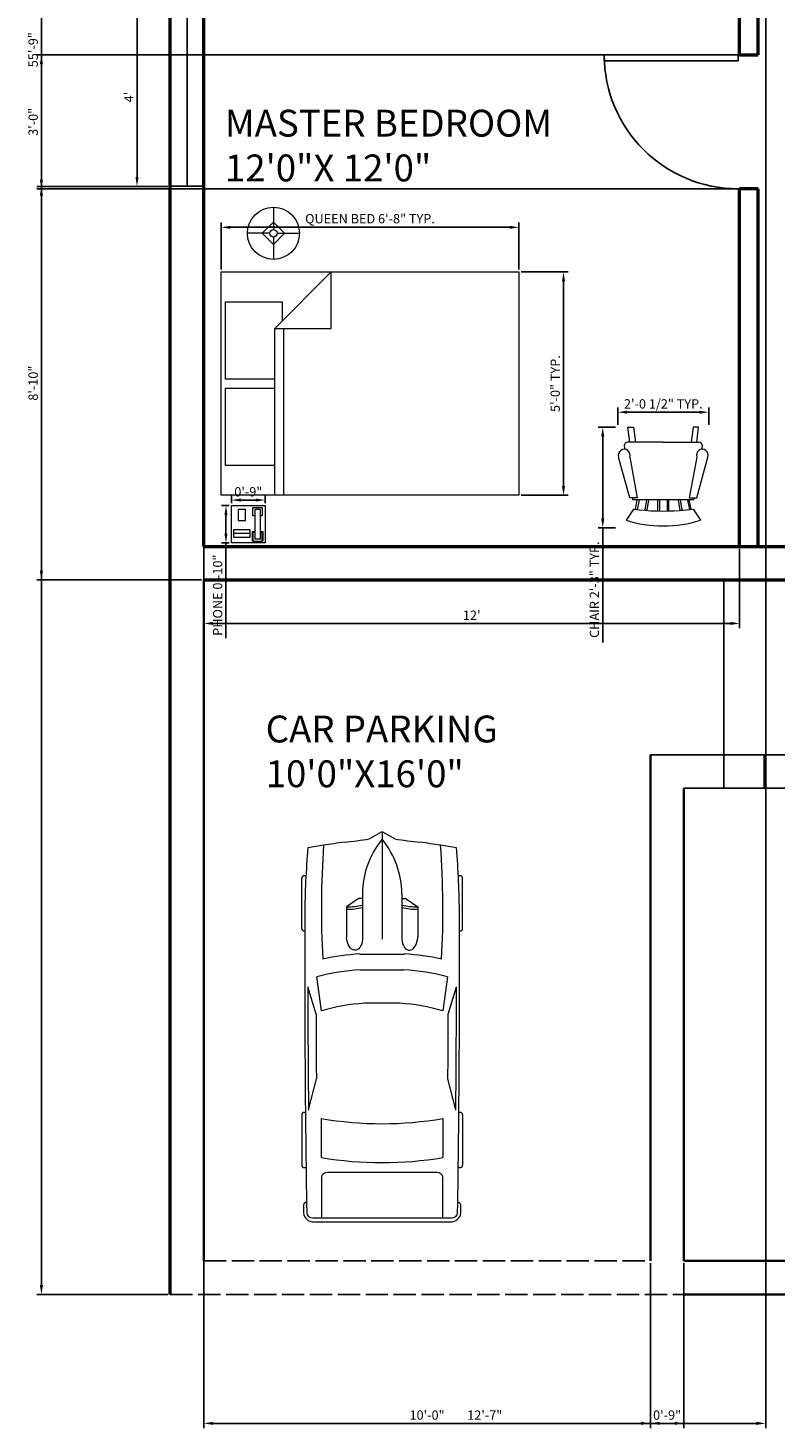
# Model space of a CAD drawing. Units: inches. Extents: x 25547 to 25983, y 30413 to 31159.
# Tile 1 of 5: x 25549 to 25750, y 30414 to 30790. Entities that reach past the tile are written whole.
import ezdxf

# ---------------------------------------------------------------- set-up
doc = ezdxf.new("R2010")
doc.units = ezdxf.units.IN
doc.linetypes.add('ACAD_ISO02W100', pattern=[15, 12, -3])
for name, color, linetype, lineweight in [('A-AREA-IDEN', 11, 'Continuous', 25), ('A-EQPM', 6, 'Continuous', 18), ('A-FLOR-PORC', 151, 'Continuous', 25), ('A-WALL', 7, 'Continuous', 50), ('C-PARK-ENTR', 7, 'ACAD_ISO02W100', 25), ('CAR', 20, 'Continuous', 13), ('DIM', 4, 'Continuous', 18), ('DOOR', 3, 'Continuous', 25), ('FURNITURES', 6, 'Continuous', 18), ('L-SITE-WALL', 7, 'Continuous', 35), ('WINDOW', 1, 'Continuous', 25)]:
    doc.layers.add(name, color=color, linetype=linetype, lineweight=lineweight)
doc.styles.get("Standard").update_dxf_attribs({"font": 'arial.ttf'})
doc.dimstyles.new('ISO-25', dxfattribs={"dimtxt": 2.5, "dimasz": 2.5, "dimexe": 1.25, "dimexo": 0.625, "dimtad": 1, "dimlunit": 3, "dimtxsty": 'Standard', "dimcen": 2.5, "dimadec": 0, "dimazin": 0, "dimtfac": 1, "dimtmove": 0, "dimatfit": 3, "dimfxl": 1, "dimarcsym": 0})

# ---------------------------------------------------------------- blocks, each defined once
blk = doc.blocks.new('*U3')
for p, q in [((0, 0), (0, -6)), ((-40, 0), (-40, -6))]:
    blk.add_line(p, q)
blk.add_lwpolyline([(0, 0), (0, 40), (-1.75, 40), (-1.75, 0)], close=True)
blk.add_arc((0, 0), 40, 90, 180)
blk = doc.blocks.new('Phone - Desk')
for p, q in [((-4.5, -5), (-4.5, 5)), ((-4.5, 5), (4.5, 5)), ((-4, 4.5), (-4, 2)), ((-3.75, 4.5), (-3.75, 2.25)), ((-1.25, 4.5), (-3.75, 4.5)), ((-3.25, 4), (-3.25, -4)), ((-3.25, 4), (-1.75, 4)), ((-1.75, -4), (-1.75, 4)), ((-1.25, 2.25), (-1.25, 4.5)), ((-1, 2), (-1, 4.5)), ((4.5, 5), (4.5, -5)), ((-4, 2), (-3.25, 2)), ((-3.75, 2.25), (-3.25, 2.25)), ((-1.75, 2.25), (-1.25, 2.25)), ((-1.75, 2), (-1, 2)), ((4, 3.5), (-0.5, 3.5)), ((-0.5, 3.5), (-0.5, 1.5)), ((-0.5, 2.5), (4, 2.5)), ((-0.5, 1.5), (4, 1.5)), ((4, 1.5), (4, 3.5)), ((-3.75, -2.25), (-3.25, -2.25)), ((-3.75, -4.5), (-3.75, -2.25)), ((-1.75, -2.25), (-1.25, -2.25)), ((-1.25, -2.25), (-1.25, -4.5)), ((2.75, -1), (0.75, -1)), ((0.75, -1), (0.75, -4)), ((2.75, -4), (2.75, -1)), ((4.5, -5), (-4.5, -5)), ((-1.25, -4.5), (-3.75, -4.5)), ((-3.25, -4), (-1.75, -4)), ((0.75, -4), (2.75, -4))]:
    blk.add_line(p, q)
blk = doc.blocks.new('Bed - Queen')
for p, q in [((0, -80.00003), (0, 0)), ((0, 0), (59.99999, 0)), ((59.99999, 0), (59.99999, -80.00003)), ((7.99999, -1.2), (28.79998, -1.2)), ((7.99999, -14.4), (7.99999, -1.2)), ((28.79998, -1.2), (28.79998, -14.4)), ((31.19999, -1.2), (51.99999, -1.2)), ((31.19999, -14.4), (31.19999, -1.2)), ((51.99999, -1.2), (51.99999, -16.4)), ((0, -14.4), (44.8, -14.4)), ((59.99999, -29.6), (44.8, -14.4)), ((44.8, -14.4), (44.8, -29.6)), ((44.8, -16.8), (0, -16.8)), ((51.99999, -16.4), (46.79936, -16.4)), ((44.8, -29.6), (59.99999, -29.6)), ((59.99999, -80.00003), (0, -80.00003))]:
    blk.add_line(p, q)
blk = doc.blocks.new('Lamp - Table')
for p, q in [((0, 7), (0, 1)), ((-1, 0), (-7, 0)), ((0, 3), (-3, 0)), ((-3, 0), (0, -3)), ((3, 0), (0, 3)), ((0, -3), (3, 0)), ((1, 0), (7, 0)), ((0, -1), (0, -7))]:
    blk.add_line(p, q)
for radius in [7, 1]:
    blk.add_circle((0, 0), radius)
blk = doc.blocks.new('Chair - Rocking')
for p, q in [((-8, -4.5), (-10, -1.5)), ((8, -4.5), (10, -1.5)), ((-9, -7.5), (-12, -18.49999)), ((-7, -7.5), (-9, -7.5)), ((-9, -18.49999), (-7, -7.5)), ((-8.23428, -6.99939), (-8.3093, -7.47958)), ((-8.23041, -7), (8.23915, -7)), ((-7.5, -4.5), (-7, -7)), ((-6.5, -7), (-7.02225, -4.43)), ((-4.5, -7), (-4.96674, -4.19951)), ((-4, -7), (-4.40532, -4.16272)), ((-1.5, -4.05012), (-1.5, -7)), ((-1, -7), (-1, -4.05012)), ((1, -7), (1, -4.04655)), ((1.5, -4.05012), (1.5, -7)), ((4, -7), (4.40187, -4.18694)), ((4.5, -7), (4.96761, -4.19437)), ((6.5, -7), (7, -4.4057)), ((7.5, -4.5), (7, -7)), ((7, -7.5), (9, -7.5)), ((9, -18.49999), (7, -7.5)), ((8.31071, -7.48854), (8.23449, -7.00073)), ((9, -7.5), (12, -18.49999)), ((-10.36644, -20.64523), (-10.5, -21.49999)), ((-9, -22.49999), (-9.5, -26.49999)), ((0, -22.49999), (-9.5, -22.49999)), ((-8, -26.49999), (-7.5, -22.49999)), ((0, -22.49999), (9.5, -22.49999)), ((8, -26.49999), (7.5, -22.49999)), ((9, -22.49999), (9.5, -26.49999)), ((10.5, -21.49999), (10.3575, -20.58798)), ((-9.5, -26.49999), (-8, -26.49999)), ((9.5, -26.49999), (8, -26.49999))]:
    blk.add_line(p, q)
for centre, radius, start, end in [((0, -34.08333), 34.08333, 72.93847, 107.0615), ((0, -68.25004), 64.25, 93.92211, 97.15267), ((0, -68.25004), 64.25, 82.84733, 93.92211), ((-10.5, -18.99999), 1.58114, 161.5651, 18.43495), ((10.5, -18.99999), 1.58114, 161.5651, 18.43495), ((-9.5, -21.49999), 1, 180, 270), ((9.5, -21.49999), 1, 270, 0)]:
    blk.add_arc(centre, radius, start, end)
blk = doc.blocks.new('*D26')
at = {"layer": 'Defpoints', "color": 0, "transparency": 16777216}
for p in [(25587.53, 30795.61), (25578.58, 30747.61), (25587.53, 30747.61)]:
    blk.add_point(p, dxfattribs=at)
at = {"layer": 'DIM', "color": 0, "lineweight": -2, "transparency": 16777216}
for p, q in [((25586.9, 30795.61), (25577.33, 30795.61)), ((25578.58, 30793.11), (25578.58, 30750.11)), ((25586.9, 30747.61), (25577.33, 30747.61))]:
    blk.add_line(p, q, dxfattribs=at)
at = {"layer": 'DIM', "color": 0, "transparency": 16777216}
for points in [[(25578.17, 30793.11), (25579, 30793.11), (25578.58, 30795.61)], [(25578.17, 30750.11), (25579, 30750.11), (25578.58, 30747.61)]]:
    blk.add_solid(points, dxfattribs=at)
at = {"layer": 'DIM', "color": 0, "transparency": 16777216, "insert": (25576.71, 30771.61), "char_height": 2.5, "attachment_point": 5, "rotation": 90}
blk.add_mtext("4'", dxfattribs=at)
blk = doc.blocks.new('*D27')
at = {"layer": 'Defpoints', "color": 0, "transparency": 16777216}
for p in [(25596.53, 30650.83), (25740.53, 30650.83), (25740.53, 30630.15)]:
    blk.add_point(p, dxfattribs=at)
at = {"layer": 'DIM', "color": 0, "lineweight": -2, "transparency": 16777216}
for p, q in [((25596.53, 30650.2), (25596.53, 30628.9)), ((25740.53, 30650.2), (25740.53, 30628.9)), ((25599.03, 30630.15), (25738.03, 30630.15))]:
    blk.add_line(p, q, dxfattribs=at)
at = {"layer": 'DIM', "color": 0, "transparency": 16777216}
for points in [[(25599.03, 30630.57), (25599.03, 30629.74), (25596.53, 30630.15)], [(25738.03, 30630.57), (25738.03, 30629.74), (25740.53, 30630.15)]]:
    blk.add_solid(points, dxfattribs=at)
at = {"layer": 'DIM', "color": 0, "transparency": 16777216, "insert": (25668.53, 30632.03), "char_height": 2.5, "attachment_point": 5}
blk.add_mtext("12'", dxfattribs=at)
blk = doc.blocks.new('*U35')
for p, q in [((21.1, 37.41), (21.1, 36.83)), ((46.55, 38.89), (22.35, 38.89)), ((47.8, 37.39), (47.8, 37.41)), ((87.99, 31.87), (74.76, 35.92)), ((134.31, 35.6), (119.29, 31.78)), ((135.45, 37.07), (135.45, 37.41)), ((136.7, 38.89), (160.9, 38.89)), ((162.15, 37.41), (162.15, 36.77)), ((70.03, 31.54), (86.41, 29.35)), ((138.42, 29.35), (157.25, 29.35)), ((186.47, 29.35), (167.01, 29.35)), ((186.47, -33.5), (186.47, 33.5)), ((188.4, -32.76), (188.4, 32.76)), ((164.52, 26.39), (164.52, -26.39)), ((32.27, 11.63), (36.13, 17.17)), ((36.13, 17.17), (50.94, 17.17)), ((29.77, 9.51), (51.68, 9.51)), ((32.12, 9.51), (32.12, 11.15)), ((58.92, -10.77), (58.92, 10.77)), ((66.55, -10.53), (66.55, 10.53)), ((82.74, 8.5), (82.74, -8.5)), ((186.47, -10.53), (186.47, 10.53)), ((3.27, 6.13), (0.1, 0.41)), ((0, 0), (51.68, 0)), ((0.1, -0.41), (3.27, -6.13)), ((29.77, -9.51), (51.68, -9.51)), ((32.12, -9.51), (32.12, -11.15)), ((32.27, -11.63), (36.13, -17.17)), ((36.13, -17.17), (50.94, -17.17)), ((86.41, -29.35), (70.03, -31.54)), ((87.99, -31.87), (74.76, -35.92)), ((134.31, -35.6), (119.29, -31.78)), ((157.25, -29.35), (138.42, -29.35)), ((167.01, -29.35), (186.47, -29.35)), ((21.1, -37.41), (21.1, -36.83)), ((46.55, -38.89), (22.35, -38.89)), ((47.8, -37.39), (47.8, -37.41)), ((135.45, -37.07), (135.45, -37.41)), ((136.7, -38.89), (160.9, -38.89)), ((162.15, -37.41), (162.15, -36.77))]:
    blk.add_line(p, q)
for centre, major_axis, ratio, start_param, end_param in [((266.03, -27.52), (0, 313.31), 0.842304, 1.367076, 1.39176), ((41.19, -490.86), (0, 528.23), 0.842304, 0.00281, 0.075598), ((22.35, 37.41), (0, -1.48), 0.842304, 3.141593, 4.712389), ((64.48, -10555.62), (0, 10593.03), 0.842304, -0.013397, 0.002797), ((46.55, 37.41), (0, 1.48), 0.842304, -1.570796, 0), ((64.48, -10555.62), (0, -10591.55), 0.842304, 3.133765, 3.140441), ((136.7, 37.41), (0, -1.48), 0.842304, 3.141593, 4.712389), ((160.9, 37.41), (0, 1.48), 0.842304, -1.570796, 0), ((180.63, 35.84), (0, 2.22), 0.842304, -0.013017, 1.249894), ((64.48, -10556.36), (0, 10595.31), 0.842304, -0.013397, -0.013017), ((183.98, 33.5), (0, -2.96), 0.842304, 1.570796, 3.128196), ((183.98, 32.76), (0, -5.25), 0.842304, 1.570796, 3.128196), ((259.18, -27.52), (0, -305.3), 0.842304, 4.528606, 4.561838), ((37.47, -593.96), (0, -623.33), 0.842304, 3.096046, 3.200911), ((134.4, 5.39), (0, -89.78), 0.842304, 4.449482, 4.652344), ((135.29, 5.39), (0, 81.77), 0.842304, 1.245306, 1.50788), ((149.6, 2.8), (0, -79.58), 0.842304, 4.372215, 4.640744), ((95.79, -3666.35), (0, -3698.24), 0.842304, 3.134049, 3.144098), ((17.08, 0), (0, 147.02), 0.842304, 4.511394, 4.913384), ((35.91, 0), (0, 147.02), 0.842304, 4.511394, 4.913384), ((167.01, 26.39), (0, 2.96), 0.842304, 0, 1.570796), ((-204.49, 52.4), (0, -250.96), 0.842304, 1.385369, 1.434372), ((13.04, 17.01), (0, 27.42), 0.842304, 4.435146, 4.718221), ((14.2, 17.01), (0, 27.42), 0.842304, 4.435146, 4.718221), ((50.79, 13.34), (6.34, -0.36), 0.603834, -1.395552, 1.581315), ((29.77, -46.66), (0, 56.17), 0.842304, 0, 0.590319), ((32.75, 11.15), (0, 0.74), 0.842304, 0.879714, 1.570796), ((0.62, 0), (0, -0.74), 0.842304, 4.131459, 5.293319), ((-204.49, -52.4), (0, 250.96), 0.842304, -1.434372, -1.385369), ((29.77, 46.66), (0, 56.17), 0.842304, 2.551274, 3.141593), ((32.75, -11.15), (0, -0.74), 0.842304, 4.712389, 5.403472), ((13.04, -17.01), (0, -27.42), 0.842304, 1.564964, 1.848039), ((14.2, -17.01), (0, -27.42), 0.842304, 1.564964, 1.848039), ((134.4, -5.39), (0, -89.78), 0.842304, -1.510751, -1.307889), ((135.29, -5.39), (0, -81.77), 0.842304, -1.50788, -1.245306), ((149.6, -2.8), (0, -79.58), 0.842304, -1.499151, -1.230623), ((259.18, 27.52), (0, 305.3), 0.842304, 1.721348, 1.754579), ((167.01, -26.39), (0, -2.96), 0.842304, 4.712389, 6.283185), ((266.03, 27.52), (0, 313.31), 0.842304, 1.749832, 1.774517), ((37.47, 593.96), (0, -623.33), 0.842304, -0.059319, 0.045547), ((95.79, 3666.35), (0, -3698.24), 0.842304, -0.002505, 0.007544), ((183.98, -33.5), (0, 2.96), 0.842304, 3.15499, 4.712389), ((183.98, -32.76), (0, -5.25), 0.842304, 0.013397, 1.570796), ((41.19, 490.86), (0, -528.23), 0.842304, -0.075598, -0.00281), ((22.35, -37.41), (0, 1.48), 0.842304, 1.570796, 3.141593), ((64.48, 10555.62), (0, 10593.03), 0.842304, 3.138796, 3.15499), ((46.55, -37.41), (0, -1.48), 0.842304, 0, 1.570796), ((64.48, 10555.62), (0, -10591.55), 0.842304, 0.001152, 0.007828), ((136.7, -37.41), (0, -1.48), 0.842304, -1.570796, 0), ((160.9, -37.41), (0, 1.48), 0.842304, 3.141593, 4.712389), ((180.63, -35.84), (0, -2.22), 0.842304, -1.249894, 0.013017), ((64.48, 10556.36), (0, 10595.31), 0.842304, 3.15461, 3.15499)]:
    blk.add_ellipse(centre, major_axis=major_axis, ratio=ratio, start_param=start_param, end_param=end_param)
at = {"extrusion": (0, 0, -1)}
blk.add_ellipse((50.79, -13.34), major_axis=(6.34, 0.36), ratio=0.603834, start_param=-1.395552, end_param=1.581315, dxfattribs=at)
blk = doc.blocks.new('WIN-48IN')
blk.add_line((4.5, 48), (4.5, 0))
blk.add_lwpolyline([(0, 48), (9, 48), (9, 0), (0, 0)], close=True)
blk = doc.blocks.new('*D40')
at = {"layer": 'Defpoints', "color": 0, "transparency": 16777216}
for p in [(25707.79, 30682.86), (25703.74, 30655.86), (25707.79, 30655.86)]:
    blk.add_point(p, dxfattribs=at)
at = {"layer": 'DIM', "color": 0, "lineweight": -2, "transparency": 16777216}
for p, q in [((25707.16, 30682.86), (25702.49, 30682.86)), ((25703.74, 30680.36), (25703.74, 30658.36)), ((25707.16, 30655.86), (25702.49, 30655.86)), ((25703.74, 30655.86), (25703.74, 30625.07))]:
    blk.add_line(p, q, dxfattribs=at)
at = {"layer": 'DIM', "color": 0, "transparency": 16777216}
for points in [[(25703.32, 30680.36), (25704.15, 30680.36), (25703.74, 30682.86)], [(25703.32, 30658.36), (25704.15, 30658.36), (25703.74, 30655.86)]]:
    blk.add_solid(points, dxfattribs=at)
at = {"layer": 'DIM', "color": 0, "transparency": 16777216, "insert": (25701.82, 30639.22), "char_height": 2.5, "attachment_point": 5, "rotation": 90}
blk.add_mtext('CHAIR 2\'-3" TYP.', dxfattribs=at)
blk = doc.blocks.new('*D41')
at = {"layer": 'Defpoints', "color": 0, "transparency": 16777216}
for p in [(25707.79, 30686.91), (25707.79, 30682.86), (25732.22, 30682.86)]:
    blk.add_point(p, dxfattribs=at)
at = {"layer": 'DIM', "color": 0, "lineweight": -2, "transparency": 16777216}
for p, q in [((25707.79, 30683.49), (25707.79, 30688.16)), ((25729.72, 30686.91), (25710.29, 30686.91)), ((25732.22, 30683.49), (25732.22, 30688.16))]:
    blk.add_line(p, q, dxfattribs=at)
at = {"layer": 'DIM', "color": 0, "transparency": 16777216}
for points in [[(25710.29, 30687.33), (25710.29, 30686.5), (25707.79, 30686.91)], [(25729.72, 30687.33), (25729.72, 30686.5), (25732.22, 30686.91)]]:
    blk.add_solid(points, dxfattribs=at)
at = {"layer": 'DIM', "color": 0, "transparency": 16777216, "insert": (25720.01, 30688.83), "char_height": 2.5, "attachment_point": 5}
blk.add_mtext('2\'-0 1/2" TYP.', dxfattribs=at)
blk = doc.blocks.new('*D44')
at = {"layer": 'Defpoints', "color": 0, "transparency": 16777216}
for p in [(25601.19, 30736.6), (25601.19, 30724.6), (25681.19, 30724.6)]:
    blk.add_point(p, dxfattribs=at)
at = {"layer": 'DIM', "color": 0, "lineweight": -2, "transparency": 16777216}
for p, q in [((25601.19, 30725.22), (25601.19, 30737.85)), ((25681.19, 30725.22), (25681.19, 30737.85)), ((25678.69, 30736.6), (25603.69, 30736.6))]:
    blk.add_line(p, q, dxfattribs=at)
at = {"layer": 'DIM', "color": 0, "transparency": 16777216}
for points in [[(25603.69, 30737.01), (25603.69, 30736.18), (25601.19, 30736.6)], [(25678.69, 30737.01), (25678.69, 30736.18), (25681.19, 30736.6)]]:
    blk.add_solid(points, dxfattribs=at)
at = {"layer": 'DIM', "color": 0, "transparency": 16777216, "insert": (25641.19, 30738.59), "char_height": 2.5, "attachment_point": 5}
blk.add_mtext('QUEEN BED 6\'-8" TYP.', dxfattribs=at)
blk = doc.blocks.new('*D45')
at = {"layer": 'Defpoints', "color": 0, "transparency": 16777216}
for p in [(25681.19, 30724.6), (25693.19, 30724.6), (25681.19, 30664.6)]:
    blk.add_point(p, dxfattribs=at)
at = {"layer": 'DIM', "color": 0, "lineweight": -2, "transparency": 16777216}
for p, q in [((25681.81, 30724.6), (25694.44, 30724.6)), ((25693.19, 30667.1), (25693.19, 30722.1)), ((25681.81, 30664.6), (25694.44, 30664.6))]:
    blk.add_line(p, q, dxfattribs=at)
at = {"layer": 'DIM', "color": 0, "transparency": 16777216}
for points in [[(25692.77, 30722.1), (25693.61, 30722.1), (25693.19, 30724.6)], [(25692.77, 30667.1), (25693.61, 30667.1), (25693.19, 30664.6)]]:
    blk.add_solid(points, dxfattribs=at)
at = {"layer": 'DIM', "color": 0, "transparency": 16777216, "insert": (25691.29, 30694.6), "char_height": 2.5, "attachment_point": 5, "rotation": 90}
blk.add_mtext('5\'-0" TYP.', dxfattribs=at)
blk = doc.blocks.new('*D66')
at = {"layer": 'Defpoints', "color": 0, "transparency": 16777216}
for p in [(25603.99, 30661.8), (25602.49, 30651.8), (25603.99, 30651.8)]:
    blk.add_point(p, dxfattribs=at)
at = {"layer": 'DIM', "color": 0, "lineweight": -2, "transparency": 16777216}
for p, q in [((25603.36, 30661.8), (25601.24, 30661.8)), ((25602.49, 30659.3), (25602.49, 30654.3)), ((25603.36, 30651.8), (25601.24, 30651.8)), ((25602.49, 30651.8), (25602.49, 30626.2))]:
    blk.add_line(p, q, dxfattribs=at)
at = {"layer": 'DIM', "color": 0, "transparency": 16777216}
for points in [[(25602.07, 30659.3), (25602.9, 30659.3), (25602.49, 30661.8)], [(25602.07, 30654.3), (25602.9, 30654.3), (25602.49, 30651.8)]]:
    blk.add_solid(points, dxfattribs=at)
at = {"layer": 'DIM', "color": 0, "transparency": 16777216, "insert": (25600.57, 30637.75), "char_height": 2.5, "attachment_point": 5, "rotation": 90}
blk.add_mtext('PHONE 0\'-10"', dxfattribs=at)
blk = doc.blocks.new('*D67')
at = {"layer": 'Defpoints', "color": 0, "transparency": 16777216}
for p in [(25603.99, 30663.3), (25603.99, 30661.8), (25612.99, 30661.8)]:
    blk.add_point(p, dxfattribs=at)
at = {"layer": 'DIM', "color": 0, "lineweight": -2, "transparency": 16777216}
for p, q in [((25603.99, 30662.43), (25603.99, 30664.55)), ((25610.49, 30663.3), (25606.49, 30663.3)), ((25612.99, 30662.43), (25612.99, 30664.55))]:
    blk.add_line(p, q, dxfattribs=at)
at = {"layer": 'DIM', "color": 0, "transparency": 16777216}
for points in [[(25606.49, 30663.72), (25606.49, 30662.89), (25603.99, 30663.3)], [(25610.49, 30663.72), (25610.49, 30662.89), (25612.99, 30663.3)]]:
    blk.add_solid(points, dxfattribs=at)
at = {"layer": 'DIM', "color": 0, "transparency": 16777216, "insert": (25608.49, 30665.2), "char_height": 2.5, "attachment_point": 5}
blk.add_mtext('0\'-9"', dxfattribs=at)
blk = doc.blocks.new('*D68')
at = {"layer": 'Defpoints', "color": 0, "transparency": 16777216}
for p in [(25552.89, 31118.83), (25587.53, 31118.83), (25587.53, 30449.83)]:
    blk.add_point(p, dxfattribs=at)
at = {"layer": 'DIM', "color": 0, "lineweight": -2, "transparency": 16777216}
for p, q in [((25586.9, 31118.83), (25551.64, 31118.83)), ((25552.89, 30452.33), (25552.89, 31116.33)), ((25586.9, 30449.83), (25551.64, 30449.83))]:
    blk.add_line(p, q, dxfattribs=at)
at = {"layer": 'DIM', "color": 0, "transparency": 16777216}
for points in [[(25552.47, 31116.33), (25553.31, 31116.33), (25552.89, 31118.83)], [(25552.47, 30452.33), (25553.31, 30452.33), (25552.89, 30449.83)]]:
    blk.add_solid(points, dxfattribs=at)
at = {"layer": 'DIM', "color": 0, "transparency": 16777216, "insert": (25550.99, 30784.33), "char_height": 2.5, "attachment_point": 5, "rotation": 90}
blk.add_mtext('55\'-9"', dxfattribs=at)
blk = doc.blocks.new('*D71')
at = {"layer": 'Defpoints', "color": 0, "transparency": 16777216}
for p in [(25596.53, 30458.83), (25716.53, 30458.83), (25716.53, 30415.19)]:
    blk.add_point(p, dxfattribs=at)
at = {"layer": 'DIM', "color": 0, "lineweight": -2, "transparency": 16777216}
for p, q in [((25596.53, 30458.2), (25596.53, 30413.94)), ((25716.53, 30458.2), (25716.53, 30413.94)), ((25599.03, 30415.19), (25714.03, 30415.19))]:
    blk.add_line(p, q, dxfattribs=at)
at = {"layer": 'DIM', "color": 0, "transparency": 16777216}
for points in [[(25599.03, 30415.61), (25599.03, 30414.77), (25596.53, 30415.19)], [(25714.03, 30415.61), (25714.03, 30414.77), (25716.53, 30415.19)]]:
    blk.add_solid(points, dxfattribs=at)
at = {"layer": 'DIM', "color": 0, "transparency": 16777216, "insert": (25656.53, 30417.09), "char_height": 2.5, "attachment_point": 5}
blk.add_mtext('10\'-0"', dxfattribs=at)
blk = doc.blocks.new('*D72')
at = {"layer": 'Defpoints', "color": 0, "transparency": 16777216}
for p in [(25716.53, 30458.83), (25725.53, 30458.83), (25725.53, 30415.19)]:
    blk.add_point(p, dxfattribs=at)
at = {"layer": 'DIM', "color": 0, "lineweight": -2, "transparency": 16777216}
for p, q in [((25716.53, 30458.2), (25716.53, 30413.94)), ((25725.53, 30458.2), (25725.53, 30413.94)), ((25719.03, 30415.19), (25723.03, 30415.19))]:
    blk.add_line(p, q, dxfattribs=at)
at = {"layer": 'DIM', "color": 0, "transparency": 16777216}
for points in [[(25719.03, 30415.61), (25719.03, 30414.77), (25716.53, 30415.19)], [(25723.03, 30415.61), (25723.03, 30414.77), (25725.53, 30415.19)]]:
    blk.add_solid(points, dxfattribs=at)
at = {"layer": 'DIM', "color": 0, "transparency": 16777216, "insert": (25721.03, 30417.09), "char_height": 2.5, "attachment_point": 5}
blk.add_mtext('0\'-9"', dxfattribs=at)
blk = doc.blocks.new('*D77')
at = {"layer": 'Defpoints', "color": 0, "transparency": 16777216}
for p in [(25596.53, 30977.83), (25747.53, 30977.83), (25747.53, 30415.19)]:
    blk.add_point(p, dxfattribs=at)
at = {"layer": 'DIM', "color": 0, "lineweight": -2, "transparency": 16777216}
for p, q in [((25596.53, 30977.2), (25596.53, 30413.94)), ((25747.53, 30977.2), (25747.53, 30413.94)), ((25599.03, 30415.19), (25745.03, 30415.19))]:
    blk.add_line(p, q, dxfattribs=at)
at = {"layer": 'DIM', "color": 0, "transparency": 16777216}
for points in [[(25599.03, 30415.61), (25599.03, 30414.77), (25596.53, 30415.19)], [(25745.03, 30415.61), (25745.03, 30414.77), (25747.53, 30415.19)]]:
    blk.add_solid(points, dxfattribs=at)
at = {"layer": 'DIM', "color": 0, "transparency": 16777216, "insert": (25672.03, 30417.07), "char_height": 2.5, "attachment_point": 5}
blk.add_mtext('12\'-7"', dxfattribs=at)
blk = doc.blocks.new('*D95')
at = {"layer": 'Defpoints', "color": 0, "transparency": 16777216}
for p in [(25587.53, 30747.61), (25552.89, 30641.83), (25596.53, 30641.83)]:
    blk.add_point(p, dxfattribs=at)
at = {"layer": 'DIM', "color": 0, "lineweight": -2, "transparency": 16777216}
for p, q in [((25586.9, 30747.61), (25551.64, 30747.61)), ((25552.89, 30745.11), (25552.89, 30644.33)), ((25595.9, 30641.83), (25551.64, 30641.83))]:
    blk.add_line(p, q, dxfattribs=at)
at = {"layer": 'DIM', "color": 0, "transparency": 16777216}
for points in [[(25552.47, 30745.11), (25553.31, 30745.11), (25552.89, 30747.61)], [(25552.47, 30644.33), (25553.31, 30644.33), (25552.89, 30641.83)]]:
    blk.add_solid(points, dxfattribs=at)
at = {"layer": 'DIM', "color": 0, "transparency": 16777216, "insert": (25550.99, 30694.72), "char_height": 2.5, "attachment_point": 5, "rotation": 90}
blk.add_mtext('8\'-10"', dxfattribs=at)
blk = doc.blocks.new('*D96')
at = {"layer": 'Defpoints', "color": 0, "transparency": 16777216}
for p in [(25552.89, 30782.94), (25745.53, 30782.94), (25745.53, 30746.94)]:
    blk.add_point(p, dxfattribs=at)
at = {"layer": 'DIM', "color": 0, "lineweight": -2, "transparency": 16777216}
for p, q in [((25744.9, 30782.94), (25551.64, 30782.94)), ((25552.89, 30749.44), (25552.89, 30780.44)), ((25744.9, 30746.94), (25551.64, 30746.94))]:
    blk.add_line(p, q, dxfattribs=at)
at = {"layer": 'DIM', "color": 0, "transparency": 16777216}
for points in [[(25552.47, 30780.44), (25553.31, 30780.44), (25552.89, 30782.94)], [(25552.47, 30749.44), (25553.31, 30749.44), (25552.89, 30746.94)]]:
    blk.add_solid(points, dxfattribs=at)
at = {"layer": 'DIM', "color": 0, "transparency": 16777216, "insert": (25550.99, 30764.94), "char_height": 2.5, "attachment_point": 5, "rotation": 90}
blk.add_mtext('3\'-0"', dxfattribs=at)

msp = doc.modelspace()

# ---------------------------------------------------------------- linework, layer by layer
at = {"layer": 'A-FLOR-PORC'}
for p, q in [((25736.247, 30641.828), (25946.557, 30641.828)), ((25736.247, 30585.868), (25736.247, 30641.828)), ((25937.528, 30594.868), (25716.528, 30594.868)), ((25937.528, 30585.868), (25725.528, 30585.868))]:
    msp.add_line(p, q, dxfattribs=at)
msp.add_lwpolyline([(25736.247, 30585.868), (25747.082, 30585.868), (25747.082, 30594.868), (25736.247, 30594.868)], close=True, dxfattribs=at)
at = {"layer": 'A-WALL'}
for p, q in [((25596.528, 30650.828), (25596.528, 31109.828)), ((25587.528, 30449.828), (25587.528, 30852.828)), ((25745.528, 30782.944), (25745.528, 30799.828)), ((25740.528, 30782.944), (25740.528, 30794.828)), ((25740.528, 30650.828), (25740.528, 30746.944)), ((25745.528, 30650.828), (25745.528, 30746.944)), ((25596.528, 30650.828), (25758.27, 30650.828)), ((25596.528, 30641.828), (25716.528, 30641.828)), ((25716.528, 30641.828), (25758.27, 30641.828))]:
    msp.add_line(p, q, dxfattribs=at)
for points in [[(25740.528, 30782.944), (25745.528, 30782.944)], [(25745.528, 30746.944), (25740.528, 30746.944)]]:
    msp.add_lwpolyline(points, dxfattribs=at)
at = {"layer": 'C-PARK-ENTR', "ltscale": 0.5}
for p, q in [((25596.528, 30458.828), (25716.528, 30458.828)), ((25587.528, 30449.828), (25725.528, 30449.828))]:
    msp.add_line(p, q, dxfattribs=at)
at = {"layer": 'L-SITE-WALL'}
for p, q in [((25596.528, 30458.828), (25596.528, 30641.828)), ((25716.528, 30458.828), (25716.528, 30594.868)), ((25725.528, 30458.828), (25725.528, 30585.868)), ((25725.528, 30458.828), (25937.528, 30458.828)), ((25725.528, 30449.828), (25946.134, 30449.828))]:
    msp.add_line(p, q, dxfattribs=at)

# ---------------------------------------------------------------- block references
at = {"layer": 'A-EQPM', "rotation": 180}
msp.add_blockref('Phone - Desk', (25608.488, 30656.802), dxfattribs=at)
at = {"layer": 'CAR', "xscale": 0.5560552358511867, "yscale": 0.5560552358511867, "zscale": 0.5560552358511867, "rotation": 270}
msp.add_blockref('*U35', (25644.455, 30574.08), dxfattribs=at)
at = {"layer": 'DOOR', "xscale": 0.9, "yscale": 0.9, "zscale": 0.9, "rotation": 90}
msp.add_blockref('*U3', (25740.128, 30782.944), dxfattribs=at)
at = {"layer": 'FURNITURES'}
msp.add_blockref('Lamp - Table', (25615.253, 30734.987), dxfattribs=at)
for name, p, rotation in [('Bed - Queen', (25601.19, 30664.596), 90), ('Chair - Rocking', (25720.005, 30656.363), 180)]:
    msp.add_blockref(name, p, dxfattribs=dict(at, rotation=rotation))
at = {"layer": 'WINDOW'}
msp.add_blockref('WIN-48IN', (25587.528, 30747.613), dxfattribs=at)

# ---------------------------------------------------------------- texts
at = {"layer": 'A-AREA-IDEN', "char_height": 7.21917, "attachment_point": 1}
for s, insert in [('{\\fArial|b1|i1|c0|p34;MASTER BEDROOM\\P12\'0"X 12\'0"}', (25602.199, 30768.196)), ('{\\fArial|b1|i1|c0|p34;CAR PARKING\\P10\'0"X16\'0"}', (25613.153, 30605.392))]:
    msp.add_mtext_dynamic_manual_height_columns(s, width=113.82935, gutter_width=18.048, heights=[0], dxfattribs=dict(at, insert=insert))

# ---------------------------------------------------------------- dimensions: what is measured, and where the dimension line sits
at = {"layer": 'DIM'}
for base, p1, p2, angle, override, picture, middle in [((25552.891, 31118.828), (25587.528, 30449.828), (25587.528, 31118.828), 90, {"dimdec": 1, "dimlfac": 1, "dimrnd": 0, "dimzin": 1, "dimdsep": 46, "dimlunit": 4, "dimfrac": 2}, '*D68', (25550.989, 30784.328)), ((25578.585, 30747.613), (25587.528, 30795.613), (25587.528, 30747.613), 90, {"dimclrd": 0, "dimclre": 0, "dimclrt": 0}, '*D26', (25576.71, 30771.613)), ((25552.891, 30782.944), (25745.528, 30746.944), (25745.528, 30782.944), 90, {"dimdec": 1, "dimlfac": 1, "dimrnd": 0, "dimzin": 1, "dimdsep": 46, "dimlunit": 4, "dimfrac": 2}, '*D96', (25550.988, 30764.944)), ((25552.891, 30641.828), (25587.528, 30747.613), (25596.528, 30641.828), 90, {"dimdec": 1, "dimlfac": 1, "dimrnd": 0, "dimzin": 1, "dimdsep": 46, "dimlunit": 4, "dimfrac": 2}, '*D95', (25550.989, 30694.721)), ((25603.988, 30663.302), (25612.988, 30661.802), (25603.988, 30661.802), 180, {"dimdec": 1, "dimlfac": 1, "dimrnd": 0, "dimzin": 1, "dimdsep": 46, "dimlunit": 4, "dimfrac": 2}, '*D67', (25608.488, 30665.204))]:
    dim = msp.add_linear_dim(base=base, p1=p1, p2=p2, angle=angle, dimstyle='ISO-25', override=override, dxfattribs=at)
    dim.commit()
    dim.dimension.update_dxf_attribs({"geometry": picture, "text_midpoint": middle})
for base, p1, p2, override, picture, middle in [((25747.528, 30415.19), (25596.528, 30977.828), (25747.528, 30977.828), {"dimdec": 1, "dimlfac": 1, "dimrnd": 0, "dimzin": 1, "dimdsep": 46, "dimlunit": 4, "dimfrac": 2}, '*D77', (25672.028, 30417.071)), ((25740.528, 30630.154), (25596.528, 30650.828), (25740.528, 30650.828), {"dimclrd": 0, "dimclre": 0, "dimclrt": 0}, '*D27', (25668.528, 30632.034)), ((25716.528, 30415.19), (25596.528, 30458.828), (25716.528, 30458.828), {"dimdec": 1, "dimlfac": 1, "dimrnd": 0, "dimzin": 1, "dimdsep": 46, "dimlunit": 4, "dimfrac": 2}, '*D71', (25656.528, 30417.092)), ((25725.528, 30415.19), (25716.528, 30458.828), (25725.528, 30458.828), {"dimdec": 1, "dimlfac": 1, "dimrnd": 0, "dimzin": 1, "dimdsep": 46, "dimlunit": 4, "dimfrac": 2}, '*D72', (25721.028, 30417.092))]:
    dim = msp.add_linear_dim(base=base, p1=p1, p2=p2, dimstyle='ISO-25', override=override, dxfattribs=at)
    dim.commit()
    dim.dimension.update_dxf_attribs({"geometry": picture, "text_midpoint": middle})
for base, p1, p2, angle, text, picture, middle in [((25601.19, 30736.596), (25681.19, 30724.596), (25601.19, 30724.596), 180, 'QUEEN BED <> TYP.', '*D44', (25641.19, 30738.591)), ((25693.19, 30724.596), (25681.19, 30664.596), (25681.19, 30724.596), 90, '<> TYP.', '*D45', (25691.288, 30694.596)), ((25707.788, 30686.913), (25732.223, 30682.863), (25707.788, 30682.863), 180, '<> TYP.', '*D41', (25720.005, 30688.831)), ((25703.738, 30655.863), (25707.788, 30682.863), (25707.788, 30655.863), 270, 'CHAIR <> TYP.', '*D40', (25701.819, 30639.215)), ((25602.488, 30651.802), (25603.988, 30661.802), (25603.988, 30651.802), 270, 'PHONE <>', '*D66', (25600.57, 30637.75))]:
    dim = msp.add_linear_dim(base=base, p1=p1, p2=p2, angle=angle, text=text, dimstyle='ISO-25', override={"dimdec": 1, "dimlfac": 1, "dimrnd": 0, "dimzin": 1, "dimdsep": 46, "dimlunit": 4, "dimfrac": 2}, dxfattribs=at)
    dim.commit()
    dim.dimension.update_dxf_attribs({"geometry": picture, "text_midpoint": middle})

doc.saveas('drawing.dxf')
